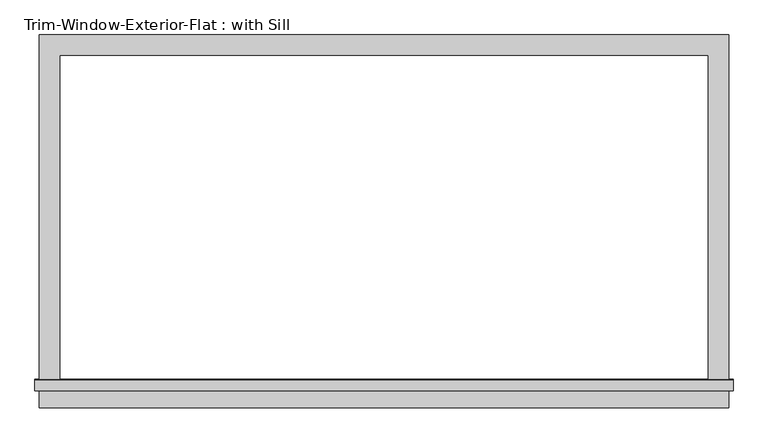
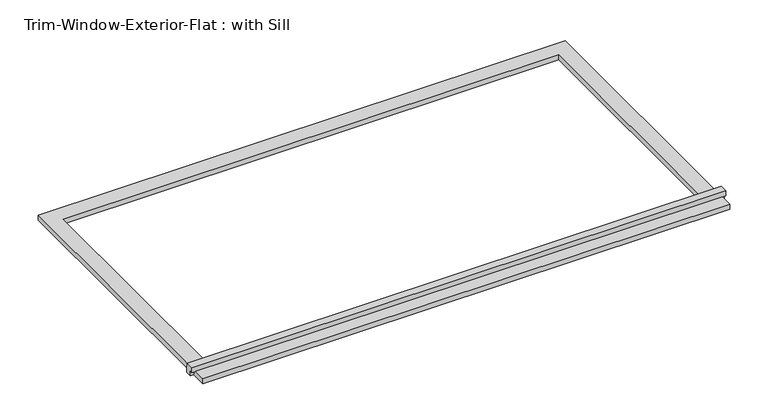
"""IFC4 building model written with IfcOpenShell, lengths in millimetres: proxy geometry, Trim-Window-Exterior-Flat : with Sill."""

from ifc_helpers import new_model, si_unit, frame, origin, origin_with_axes, place, context, project, spatial, polyline, outline, extrude, source, transform, mapped, element, save


def trim_window_exterior_flat_with_sill_3c945769(model_context):
    return source(origin(), model_context, "Body", "SweptSolid", [
        extrude(outline(polyline([(971.55, -936.5823709), (971.55, -993.7323709), (-971.55, -993.7323709), (-971.55, -936.5823709), (971.55, -936.5823709)])), origin_with_axes(), (0.0, 0.0, 1.0), 19.05),
        extrude(outline(polyline([(-946.15, 38.1), (-916.8580645, 38.1), (-914.4, 19.05), (-914.4, 0.0), (-936.5823709, 0.0), (-936.5823709, 19.05), (-946.15, 19.05), (-946.15, 38.1)])), frame((-984.25, 0.0, 0.0), z_axis=(1.0, 0.0, 0.0), x_axis=(0.0, 1.0, 0.0)), (0.0, 0.0, 1.0), 1968.5),
        extrude(outline(polyline([(-971.55, 57.15), (971.55, 57.15), (971.55, -914.4), (914.4, -914.4), (914.4, 0.0), (-914.4, 0.0), (-914.4, -914.4), (-971.55, -914.4), (-971.55, 57.15)])), origin_with_axes(), (0.0, 0.0, 1.0), 19.05),
    ])


if __name__ == "__main__":
    model = new_model("IFC4")
    model_context = context("Model", 3, world=origin())
    ifc_project = project(units=[si_unit("LENGTHUNIT", "METRE", prefix="MILLI")], contexts=[model_context])
    site = spatial("IfcSite", under=ifc_project)
    building = spatial("IfcBuilding", under=site)
    placement = place(None, origin())
    trim_window_exterior_flat_with_sill_shape = trim_window_exterior_flat_with_sill_3c945769(model_context)
    element("IfcBuildingElementProxy", 1, Name="Trim-Window-Exterior-Flat : with Sill", ObjectType="Trim-Window-Exterior-Flat : with Sill", at=placement, inside=building, context=model_context, shape_type="MappedRepresentation", body=[
        mapped(trim_window_exterior_flat_with_sill_shape, transform((0.0, 0.0, 0.0), x_axis=(1.0, 0.0, 0.0), y_axis=(0.0, 1.0, 0.0), z_axis=(0.0, 0.0, 1.0))),
    ])
    save(model, "model.ifc")

# Revit data of these elements
# Type "Trim-Window-Exterior-Flat : with Sill"
#   Trim Width = 0.1875 ft
#   Trim Thickness_Picture Frame = 0.104167 ft
#   Trim Thickness_with Sill = 0.0625 ft
#   Sill Thickness = 0.104167 ft
#   Opening Width [instance default] = 2 ft
#   Opening Height [instance default] = 3 ft
#   Default Elevation = 4 ft
#   Sill = yes
#   Picture Frame = no
#   Trim Material [instance default] = none
# Element 1 (IfcBuildingElementProxy, "Trim-Window-Exterior-Flat : with Sill")
#   Opening Width = 6 ft
#   Trim Material = Clad - White
#   Materials on its faces: "Clad - White"
# Materials
#   "Clad - White": class "Wood", colour RGB 242 242 238, transparency 0, Cost = 0
